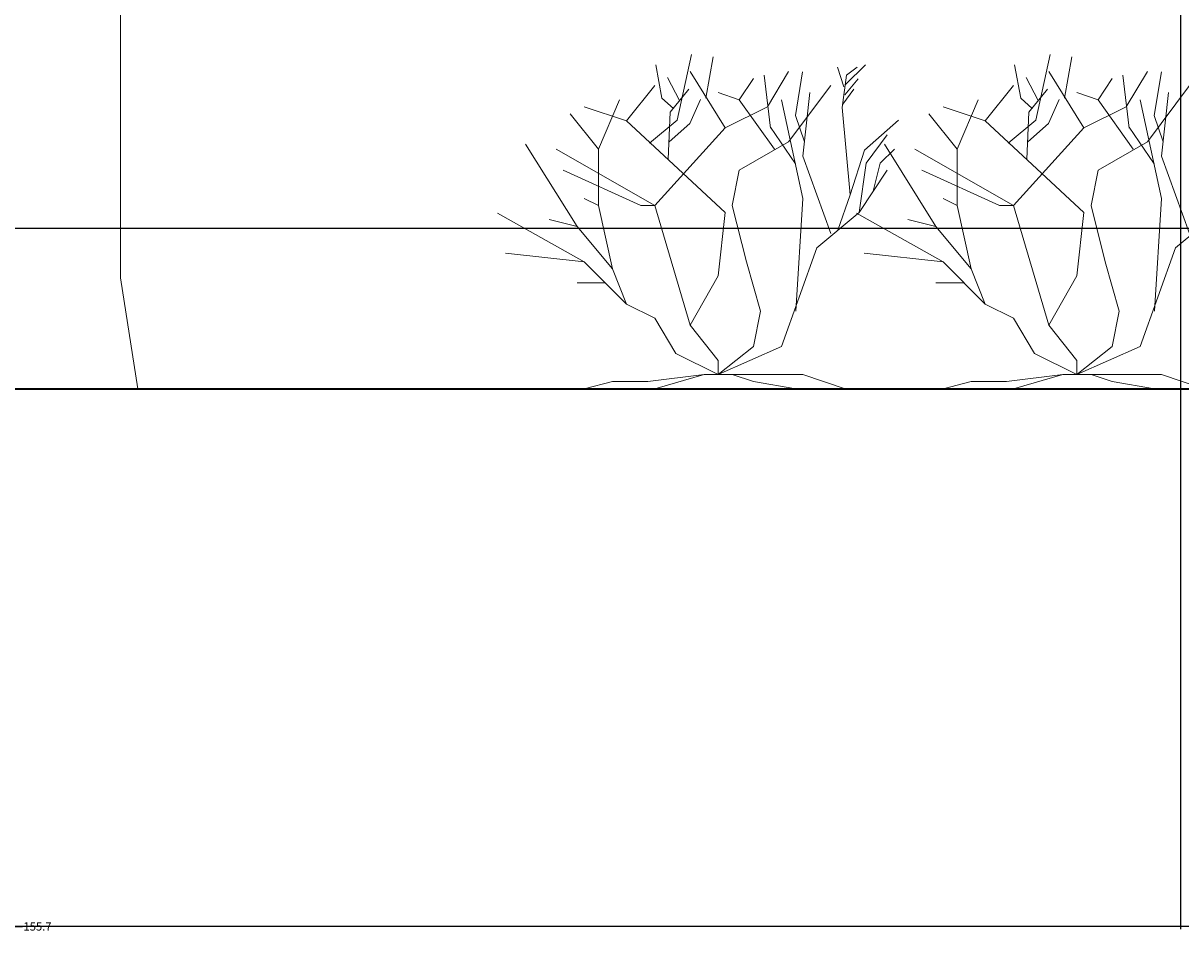
# Model space of a CAD drawing. Units: inches. Extents: x -26 to 776, y -22 to 650.
# Tile 43 of 62: x 506 to 584, y -22 to 40. Entities that reach past the tile are written whole.
import ezdxf

# ---------------------------------------------------------------- set-up
doc = ezdxf.new("R2010")
doc.units = ezdxf.units.IN
doc.header["$MEASUREMENT"] = 0
for name, color, linetype, lineweight in [('A-ANNO-DIMS', 2, 'Continuous', 18), ('C-TOPO', 7, 'Continuous', 35), ('L-PLNT-SHRB', 94, 'Continuous', 13), ('L-PLNT-TREE', 94, 'Continuous', 18)]:
    doc.layers.add(name, color=color, linetype=linetype, lineweight=lineweight)
doc.styles.get("Standard").update_dxf_attribs({"font": 'arial.ttf'})
doc.dimstyles.get("Standard").update_dxf_attribs({"dimtxt": 0.5625, "dimasz": 0.18, "dimexe": 0.18, "dimexo": 0.0625, "dimgap": 0.09, "dimtad": 0, "dimtih": 1, "dimtoh": 1, "dimdec": 4, "dimzin": 0, "dimdsep": 46, "dimlunit": 4, "dimtxsty": 'Standard', "dimcen": 0.09, "dimadec": 0, "dimazin": 0, "dimtfac": 1, "dimtdec": 4, "dimtofl": 0, "dimtmove": 0, "dimatfit": 3, "dimfxl": 1, "dimtolj": 1, "dimtzin": 0, "dimarcsym": 0})

# ---------------------------------------------------------------- blocks, each defined once
blk = doc.blocks.new('Tree - type 2 deciduous elevation')
blk.add_lwpolyline([(0.387, 23.669), (-0.576, 13.271), (-0.576, 3.686), (0, 0)])
blk = doc.blocks.new('Shrub - elevation')
for p, q in [((-11.433, 18.289), (-10.457, 22.749)), ((-9.48, 19.775), (-8.992, 22.592)), ((-12.471, 19.775), (-12.898, 22.044)), ((-8.16, 17.76), (-10.56, 21.6)), ((-5.086, 17.741), (-5.513, 21.34)), ((-5.28, 19.2), (-3.84, 21.6)), ((-3.377, 18.602), (-2.888, 21.575)), ((-0.508, 21.888), (-0.081, 20.558)), ((-0.203, 19.149), (0.102, 21.34)), ((0.041, 20.714), (1.384, 22.044)), ((0.102, 21.34), (0.835, 21.888)), ((-14.88, 18.24), (-12.96, 20.64)), ((-11.28, 19.619), (-12.104, 21.184)), ((-7.2, 19.68), (-6.24, 21.12)), ((-3.84, 16.8), (-0.96, 20.64)), ((-0.02, 20.01), (0.896, 21.105)), ((-11.677, 19.071), (-12.471, 19.775)), ((-11.921, 18.836), (-10.64, 20.401)), ((-7.2, 19.68), (-8.64, 20.16)), ((-2.88, 15.84), (-2.4, 20.16)), ((-0.142, 19.384), (0.59, 20.401)), ((-14.88, 18.24), (-17.76, 19.2)), ((-16.8, 16.32), (-15.36, 19.68)), ((-10.579, 18.054), (-9.846, 19.697)), ((-8.16, 17.76), (-5.28, 19.2)), ((-4.8, 16.32), (-7.2, 19.68)), ((-2.88, 12.96), (-4.32, 19.68)), ((0.346, 13.203), (-0.203, 19.149)), ((-16.8, 16.32), (-18.72, 18.72)), ((-8.16, 12), (-14.88, 18.24)), ((-13.325, 16.724), (-11.433, 18.289)), ((-12.043, 15.628), (-11.921, 18.836)), ((-2.766, 16.802), (-3.377, 18.602)), ((1.323, 16.254), (3.642, 18.289)), ((-12.96, 12.48), (-8.16, 17.76)), ((-11.982, 16.802), (-10.579, 18.054)), ((-3.377, 15.315), (-5.086, 17.819)), ((-18.24, 11.04), (-21.755, 16.655)), ((-7.2, 14.88), (-3.84, 16.8)), ((1.44, 15.36), (2.88, 17.28)), ((-12.96, 12.48), (-19.68, 16.32)), ((-16.8, 12.48), (-16.8, 16.32)), ((-0.96, 10.56), (-2.88, 15.84)), ((0.346, 13.203), (1.323, 16.254)), ((2.4, 15.36), (3.36, 16.32)), ((0.96, 12), (1.44, 15.36)), ((1.92, 13.44), (2.4, 15.36)), ((-13.92, 12.48), (-19.2, 14.88)), ((-7.68, 12.48), (-7.2, 14.88)), ((0.96, 12), (2.88, 14.88)), ((-16.8, 12.48), (-17.76, 12.96)), ((-3.36, 5.28), (-2.88, 12.96)), ((-0.48, 10.8), (0.346, 13.203)), ((-17.76, 8.64), (-23.663, 11.961)), ((-15.84, 8.16), (-16.8, 12.48)), ((-12.96, 12.48), (-13.92, 12.48)), ((-10.56, 4.32), (-12.96, 12.48)), ((-8.64, 7.68), (-8.16, 12)), ((-6.72, 8.64), (-7.68, 12.48)), ((-1.92, 9.6), (0.96, 12)), ((-18.24, 11.04), (-20.16, 11.52)), ((-15.84, 8.16), (-18.24, 11.04)), ((-4.32, 2.88), (-1.92, 9.6)), ((-17.76, 8.64), (-23.128, 9.222)), ((-14.88, 5.76), (-17.76, 8.64)), ((-14.88, 5.76), (-15.84, 8.16)), ((-5.76, 5.28), (-6.72, 8.64)), ((-16.32, 7.2), (-18.24, 7.2)), ((-10.56, 4.32), (-8.64, 7.68)), ((-12.96, 4.8), (-14.88, 5.76)), ((-11.52, 2.4), (-12.96, 4.8)), ((-6.24, 2.88), (-5.76, 5.28)), ((-8.64, 1.92), (-10.56, 4.32)), ((-8.64, 0.96), (-11.52, 2.4)), ((-8.64, 0.96), (-4.32, 2.88)), ((-8.64, 0.96), (-6.24, 2.88)), ((-8.64, 0.96), (-8.64, 1.92)), ((-9.6, 0.96), (-13.44, 0.48)), ((-9.6, 0.96), (-12.96, 0)), ((-9.6, 0.96), (-7.68, 0.96)), ((-8.64, 0.96), (-2.88, 0.96)), ((-7.68, 0.96), (-6.24, 0.48)), ((-2.88, 0.96), (0, 0)), ((-15.84, 0.48), (-17.76, 0)), ((-13.44, 0.48), (-15.84, 0.48)), ((-6.24, 0.48), (-3.36, 0))]:
    blk.add_line(p, q)
blk = doc.blocks.new('*D13')
at = {"layer": 'A-ANNO-DIMS', "color": 0, "lineweight": -2, "transparency": 16777216}
for p, q in [((738.75, 50.786), (738.75, -21.315)), ((11.107, 15.42), (11.107, -21.315)), ((11.287, -21.135), (373.892, -21.135)), ((738.57, -21.135), (375.965, -21.135))]:
    blk.add_line(p, q, dxfattribs=at)
at = {"layer": 'A-ANNO-DIMS', "color": 0, "transparency": 16777216}
for points in [[(11.287, -21.105), (11.287, -21.165), (11.107, -21.135)], [(738.57, -21.105), (738.57, -21.165), (738.75, -21.135)]]:
    blk.add_solid(points, dxfattribs=at)
at = {"layer": 'Defpoints', "color": 0, "transparency": 16777216}
for p in [(738.75, 50.848), (11.107, 15.482), (738.75, -21.135)]:
    blk.add_point(p, dxfattribs=at)
at = {"layer": 'A-ANNO-DIMS', "color": 0, "transparency": 16777216, "insert": (374.929, -21.135), "char_height": 0.5625, "attachment_point": 5}
blk.add_mtext('\\A1;727.6', dxfattribs=at)
blk = doc.blocks.new('*D20')
at = {"layer": 'A-ANNO-DIMS', "color": 0, "lineweight": -2, "transparency": 16777216}
for p, q in [((425.806, 455.472), (775.335, 455.472)), ((775.155, 455.292), (775.155, 235.854)), ((775.155, 15.662), (775.155, 235.1)), ((425.806, 15.482), (775.335, 15.482))]:
    blk.add_line(p, q, dxfattribs=at)
at = {"layer": 'A-ANNO-DIMS', "color": 0, "transparency": 16777216}
for points in [[(775.125, 455.292), (775.185, 455.292), (775.155, 455.472)], [(775.125, 15.662), (775.185, 15.662), (775.155, 15.482)]]:
    blk.add_solid(points, dxfattribs=at)
at = {"layer": 'Defpoints', "color": 0, "transparency": 16777216}
for p in [(425.743, 455.472), (775.155, 455.472), (425.743, 15.482)]:
    blk.add_point(p, dxfattribs=at)
at = {"layer": 'A-ANNO-DIMS', "color": 0, "transparency": 16777216, "insert": (775.155, 235.477), "char_height": 0.5625, "attachment_point": 5}
blk.add_mtext('\\A1;440', dxfattribs=at)
blk = doc.blocks.new('*D30')
at = {"layer": 'A-ANNO-DIMS', "color": 0, "lineweight": -2, "transparency": 16777216}
for p, q in [((280.68, 144.836), (775.335, 144.836)), ((775.155, 144.656), (775.155, 86.007)), ((775.155, 26.604), (775.155, 85.253)), ((280.68, 26.424), (775.335, 26.424))]:
    blk.add_line(p, q, dxfattribs=at)
at = {"layer": 'A-ANNO-DIMS', "color": 0, "transparency": 16777216}
for points in [[(775.125, 144.656), (775.185, 144.656), (775.155, 144.836)], [(775.125, 26.604), (775.185, 26.604), (775.155, 26.424)]]:
    blk.add_solid(points, dxfattribs=at)
at = {"layer": 'Defpoints', "color": 0, "transparency": 16777216}
for p in [(280.617, 144.836), (775.155, 144.836), (280.617, 26.424)]:
    blk.add_point(p, dxfattribs=at)
at = {"layer": 'A-ANNO-DIMS', "color": 0, "transparency": 16777216, "insert": (775.155, 85.63), "char_height": 0.5625, "attachment_point": 5}
blk.add_mtext('\\A1;118.41', dxfattribs=at)
blk = doc.blocks.new('*D38')
at = {"layer": 'A-ANNO-DIMS', "color": 0, "lineweight": -2, "transparency": 16777216}
for p, q in [((280.68, 26.424), (775.335, 26.424)), ((775.155, 26.244), (775.155, 21.33)), ((775.155, 15.662), (775.155, 20.576)), ((289.305, 15.482), (775.335, 15.482))]:
    blk.add_line(p, q, dxfattribs=at)
at = {"layer": 'A-ANNO-DIMS', "color": 0, "transparency": 16777216}
for points in [[(775.125, 26.244), (775.185, 26.244), (775.155, 26.424)], [(775.125, 15.662), (775.185, 15.662), (775.155, 15.482)]]:
    blk.add_solid(points, dxfattribs=at)
at = {"layer": 'Defpoints', "color": 0, "transparency": 16777216}
for p in [(280.617, 26.424), (775.155, 26.424), (289.242, 15.482)]:
    blk.add_point(p, dxfattribs=at)
at = {"layer": 'A-ANNO-DIMS', "color": 0, "transparency": 16777216, "insert": (775.155, 20.953), "char_height": 0.5625, "attachment_point": 5}
blk.add_mtext('\\A1;10.942', dxfattribs=at)
blk = doc.blocks.new('*D45')
at = {"layer": 'A-ANNO-DIMS', "color": 0, "lineweight": -2, "transparency": 16777216}
for p, q in [((507.738, 408.639), (775.335, 408.639)), ((775.155, 408.459), (775.155, 212.438)), ((775.155, 15.662), (775.155, 211.683)), ((585.998, 15.482), (775.335, 15.482))]:
    blk.add_line(p, q, dxfattribs=at)
at = {"layer": 'A-ANNO-DIMS', "color": 0, "transparency": 16777216}
for points in [[(775.125, 408.459), (775.185, 408.459), (775.155, 408.639)], [(775.125, 15.662), (775.185, 15.662), (775.155, 15.482)]]:
    blk.add_solid(points, dxfattribs=at)
at = {"layer": 'Defpoints', "color": 0, "transparency": 16777216}
for p in [(507.676, 408.639), (775.155, 408.639), (585.935, 15.482)]:
    blk.add_point(p, dxfattribs=at)
at = {"layer": 'A-ANNO-DIMS', "color": 0, "transparency": 16777216, "insert": (775.155, 212.061), "char_height": 0.5625, "attachment_point": 5}
blk.add_mtext('\\A1;393.16', dxfattribs=at)
blk = doc.blocks.new('*D47')
at = {"layer": 'A-ANNO-DIMS', "color": 0, "lineweight": -2, "transparency": 16777216}
for p, q in [((584.343, 199.901), (584.343, -21.315)), ((428.648, 180.243), (428.648, -21.315)), ((428.828, -21.135), (505.483, -21.135)), ((584.163, -21.135), (507.508, -21.135))]:
    blk.add_line(p, q, dxfattribs=at)
at = {"layer": 'A-ANNO-DIMS', "color": 0, "transparency": 16777216}
for points in [[(428.828, -21.105), (428.828, -21.165), (428.648, -21.135)], [(584.163, -21.105), (584.163, -21.165), (584.343, -21.135)]]:
    blk.add_solid(points, dxfattribs=at)
at = {"layer": 'Defpoints', "color": 0, "transparency": 16777216}
for p in [(584.343, 199.963), (428.648, 180.305), (584.343, -21.135)]:
    blk.add_point(p, dxfattribs=at)
at = {"layer": 'A-ANNO-DIMS', "color": 0, "transparency": 16777216, "insert": (506.496, -21.135), "char_height": 0.5625, "attachment_point": 5}
blk.add_mtext('\\A1;155.7', dxfattribs=at)

msp = doc.modelspace()

# ---------------------------------------------------------------- linework, layer by layer
at = {"layer": 'C-TOPO'}
msp.add_line((425.7434, 15.4824), (677.9037, 15.4824), dxfattribs=at)

# ---------------------------------------------------------------- block references
at = {"layer": 'L-PLNT-SHRB'}
for p in [(561.5008, 15.4824), (585.9354, 15.4824)]:
    msp.add_blockref('Shrub - elevation', p, dxfattribs=at)
at = {"layer": 'L-PLNT-TREE', "xscale": 2.050905272406618, "yscale": 2.050905272406618, "zscale": 2.050905272406618}
msp.add_blockref('Tree - type 2 deciduous elevation', (513.3241, 15.4824), dxfattribs=at)

# ---------------------------------------------------------------- dimensions: what is measured, and where the dimension line sits
at = {"layer": 'A-ANNO-DIMS'}
for base, p1, p2, override, picture, middle in [((775.1553, 455.4717), (425.7434, 15.4824), (425.7434, 455.4717), {"dimdec": 0, "dimlfac": 1, "dimrnd": 0, "dimzin": 0, "dimdsep": 46, "dimlunit": 2}, '*D20', (775.1553, 235.477)), ((775.1553, 408.6389), (585.9354, 15.4824), (507.6759, 408.6389), {"dimdec": 2, "dimlfac": 1, "dimrnd": 0, "dimzin": 0, "dimdsep": 46, "dimlunit": 2}, '*D45', (775.1553, 212.0606)), ((775.1553, 144.8359), (280.6173, 26.4239), (280.6173, 144.8359), {"dimdec": 2, "dimlfac": 1, "dimrnd": 0, "dimzin": 0, "dimdsep": 46, "dimlunit": 2}, '*D30', (775.1553, 85.6299)), ((775.15535, 26.4239), (289.24236, 15.48237), (280.61732, 26.4239), {"dimdec": 3, "dimlfac": 1, "dimrnd": 0, "dimzin": 0, "dimdsep": 46, "dimlunit": 2}, '*D38', (775.15535, 20.95313))]:
    dim = msp.add_linear_dim(base=base, p1=p1, p2=p2, angle=90, dimstyle='Standard', override=override, dxfattribs=at)
    dim.commit()
    dim.dimension.update_dxf_attribs({"geometry": picture, "text_midpoint": middle})
for base, p1, p2, picture, middle in [((584.3428, -21.1349), (428.6484, 180.3054), (584.3428, 199.9634), '*D47', (506.4956, -21.1349)), ((738.7503, -21.1349), (11.1074, 15.4824), (738.7503, 50.8482), '*D13', (374.9289, -21.1349))]:
    dim = msp.add_linear_dim(base=base, p1=p1, p2=p2, dimstyle='Standard', override={"dimdec": 1, "dimlfac": 1, "dimrnd": 0, "dimzin": 0, "dimdsep": 46, "dimlunit": 2}, dxfattribs=at)
    dim.commit()
    dim.dimension.update_dxf_attribs({"geometry": picture, "text_midpoint": middle})

doc.saveas('drawing.dxf')
